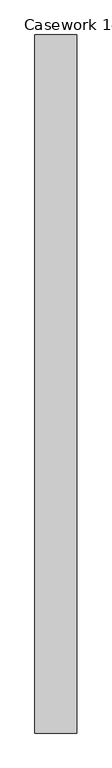
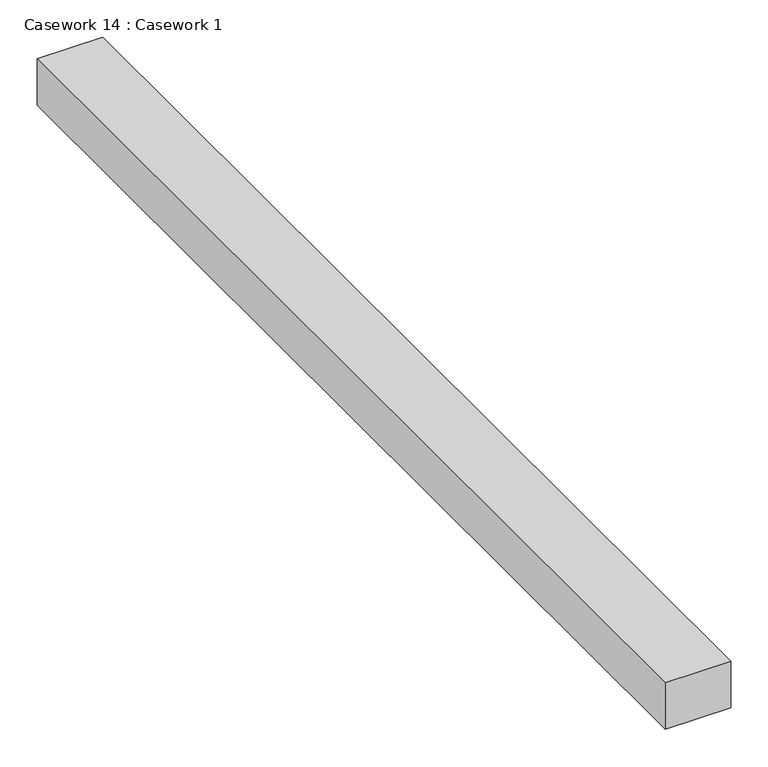
"""IFC4 building model written with IfcOpenShell, lengths in millimetres: furniture geometry, Casework 14 : Casework 1."""

from ifc_helpers import new_model, si_unit, frame, origin, place, context, project, spatial, polyline, outline, extrude, source, transform, mapped, element, save


def casework_14_casework_1_ad7f4f76(model_context):
    return source(origin(), model_context, "Body", "SweptSolid", [
        extrude(outline(polyline([(5700.1559589, 14787.9496924), (5700.1559589, 13098.8496924), (5598.5559589, 13098.8496924), (5598.5559589, 14787.9496924), (5700.1559589, 14787.9496924)])), frame((0.0, 0.0, 3581.4), z_axis=(0.0, 0.0, 1.0), x_axis=(1.0, 0.0, 0.0)), (0.0, 0.0, 1.0), 76.2),
    ])


if __name__ == "__main__":
    model = new_model("IFC4")
    model_context = context("Model", 3, world=origin())
    ifc_project = project(units=[si_unit("LENGTHUNIT", "METRE", prefix="MILLI")], contexts=[model_context])
    site = spatial("IfcSite", under=ifc_project)
    building = spatial("IfcBuilding", under=site)
    placement = place(None, origin())
    casework_14_casework_1_shape = casework_14_casework_1_ad7f4f76(model_context)
    element("IfcFurniture", 1, ObjectType="Casework 14 : Casework 1", at=placement, inside=building, context=model_context, shape_type="MappedRepresentation", body=[
        mapped(casework_14_casework_1_shape, transform((0.0, 0.0, 0.0), x_axis=(1.0, 0.0, 0.0), y_axis=(0.0, 1.0, 0.0), z_axis=(0.0, 0.0, 1.0))),
    ])
    save(model, "model.ifc")

# Revit data of these elements
# Element 1 (IfcFurniture, "Casework 14 : Casework 1")
#   Materials on its faces: "Clad - White"
# Materials
#   "Clad - White": class "Wood", colour RGB 242 242 238, transparency 0, Cost = 0
